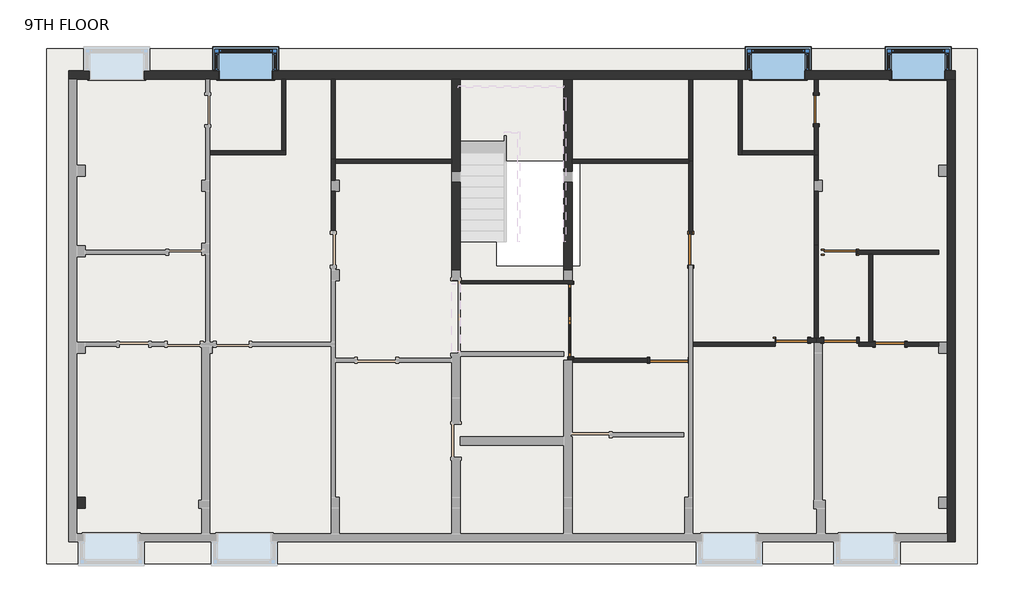
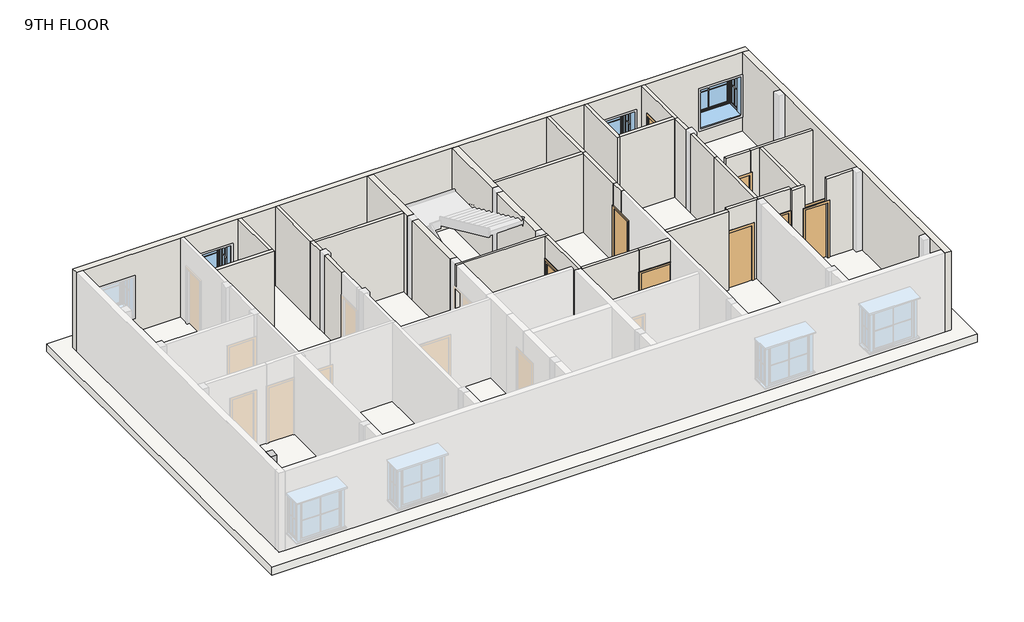
# One storey, part 2 of 3: 34 walls, 8 doors, 3 windows, 1 column, 1 slab.
"""IFC4 building model written with IfcOpenShell, lengths in millimetres."""

from ifc_helpers import new_model, si_unit, frame, origin, place, context, project, spatial, polyline, outline, extrude, faceted_brep, transform, mapped, element, save
from components import door_04ab2522, m_door_single_panel_05506f71, door_85b31ab1, door_1991e9a2, door_a431d384, door_82def9da, m_door_single_panel_3_x7_f8176753, window_19bbd869

model = new_model("IFC4")

# Units and contexts
model_context = context("Model", 3, world=origin())
ifc_project = project(units=[si_unit("LENGTHUNIT", "METRE", prefix="MILLI")], contexts=[model_context])

# Site, building, storey
site = spatial("IfcSite", under=ifc_project)
building = spatial("IfcBuilding", under=site)
storey = spatial("IfcBuildingStorey", under=building, Name="9TH FLOOR", Elevation=32004.0)

# Column
placement = place(None, origin())
element("IfcColumn", 1, ObjectType="Rectangular Column : 1'X 9\"", at=placement, inside=storey, context=model_context, shape_type="SweptSolid", body=[
    extrude(outline(polyline([(-12224.6987957, -3709.2932671), (-12224.6987957, -4014.0932671), (-12453.2987957, -4014.0932671), (-12453.2987957, -3709.2932671), (-12224.6987957, -3709.2932671)])), frame((0.0, 0.0, 32004.0), z_axis=(0.0, 0.0, 1.0), x_axis=(1.0, 0.0, 0.0)), (0.0, 0.0, 1.0), 3048.0),
])

# Doors
door_shape = door_04ab2522(model_context)
element("IfcDoor", 2, ObjectType="M_Door-Double-Glass : 6'7\"X7'", at=placement, inside=storey, context=model_context, shape_type="MappedRepresentation", body=[
    mapped(door_shape, transform((1217.5394962, 1183.3817656, 32004.0), x_axis=(0.0, 1.0, 0.0), y_axis=(-1.0, 0.0, 0.0), z_axis=(0.0, 0.0, 1.0))),
])
m_door_single_panel_shape = m_door_single_panel_05506f71(model_context)
element("IfcDoor", 3, ObjectType="M_Door-Single-Panel", at=placement, inside=storey, context=model_context, shape_type="MappedRepresentation", body=[
    mapped(m_door_single_panel_shape, transform((3933.4813133, 90.9578621, 32004.0), x_axis=(1.0, 0.0, 0.0), y_axis=(0.0, 1.0, 0.0), z_axis=(0.0, 0.0, 1.0))),
])
door_2_shape = door_85b31ab1(model_context)
element("IfcDoor", 4, ObjectType="M_Door-Single-Panel : 2'10\"X7' 2", at=placement, inside=storey, context=model_context, shape_type="MappedRepresentation", body=[
    mapped(door_2_shape, transform((4532.9512082, 3142.9626891, 32004.0), x_axis=(0.0, -1.0, 0.0), y_axis=(1.0, 0.0, 0.0), z_axis=(0.0, 0.0, 1.0))),
])
door_3_shape = door_1991e9a2(model_context)
element("IfcDoor", 5, ObjectType="M_Door-Single-Panel : 2'11\"X7' 3", at=placement, inside=storey, context=model_context, shape_type="MappedRepresentation", body=[
    mapped(door_3_shape, transform((7330.1405552, 640.4567334, 32004.0), x_axis=(1.0, 0.0, 0.0), y_axis=(0.0, 1.0, 0.0), z_axis=(0.0, 0.0, 1.0))),
])
element("IfcDoor", 6, ObjectType="M_Door-Single-Panel : 2'11\"X7' 3", at=placement, inside=storey, context=model_context, shape_type="MappedRepresentation", body=[
    mapped(door_3_shape, transform((8664.274939, 3078.8567332, 32004.0), x_axis=(-1.0, 0.0, 0.0), y_axis=(0.0, -1.0, 0.0), z_axis=(0.0, 0.0, 1.0))),
])
door_4_shape = door_a431d384(model_context)
element("IfcDoor", 7, ObjectType="M_Door-Single-Panel : 2'7\"X7' 2", at=placement, inside=storey, context=model_context, shape_type="MappedRepresentation", body=[
    mapped(door_4_shape, transform((8000.0512079, 7021.3751452, 32004.0), x_axis=(0.0, 1.0, 0.0), y_axis=(-1.0, 0.0, 0.0), z_axis=(0.0, 0.0, 1.0))),
])
door_5_shape = door_82def9da(model_context)
element("IfcDoor", 8, ObjectType="M_Door-Single-Panel : 2'8\"X7'", at=placement, inside=storey, context=model_context, shape_type="MappedRepresentation", body=[
    mapped(door_5_shape, transform((10046.0486694, 526.1567295, 32004.0), x_axis=(-1.0, 0.0, 0.0), y_axis=(0.0, -1.0, 0.0), z_axis=(0.0, 0.0, 1.0))),
])
m_door_single_panel_3_x7_shape = m_door_single_panel_3_x7_f8176753(model_context)
element("IfcDoor", 9, ObjectType="M_Door-Single-Panel : 3'X7'", at=placement, inside=storey, context=model_context, shape_type="MappedRepresentation", body=[
    mapped(m_door_single_panel_3_x7_shape, transform((8666.8012079, 640.4567334, 32004.0), x_axis=(-1.0, 0.0, 0.0), y_axis=(0.0, -1.0, 0.0), z_axis=(0.0, 0.0, 1.0))),
])

# Slab
element("IfcSlab", 10, ObjectType="Generic - 12\"", at=placement, inside=storey, context=model_context, shape_type="SweptSolid", body=[
    extrude(outline(polyline([(12464.1012075, 8698.6067329), (12464.1012075, -5550.7932662), (-13291.4987957, -5550.7932662), (-13291.4987957, 8698.6067329), (12464.1012075, 8698.6067329)]), holes=[polyline([(1456.6270108, 2700.0220048), (1456.6270108, 5595.6220048), (-829.3729892, 5595.6220048), (-829.3729892, 2700.0220048), (1456.6270108, 2700.0220048)])]), frame((0.0, 0.0, 31699.2), z_axis=(0.0, 0.0, 1.0), x_axis=(1.0, 0.0, 0.0)), (0.0, 0.0, 1.0), 304.8),
])

# Walls
element("IfcWall", 11, ObjectType="3.5\"", at=placement, inside=storey, context=model_context, shape_type="Brep", body=[
    faceted_brep([(1272.3082462, 2196.2067742, 35052.0), (1158.0082462, 2196.2067742, 35052.0), (-1848.7987998, 2196.2067742, 35052.0), (-2077.3987998, 2196.2067742, 35052.0), (-2077.3987998, 2196.2067742, 34137.6), (-1848.7987998, 2196.2067742, 34137.6), (-1848.7987998, 2196.2067742, 32004.0), (1158.0082462, 2196.2067742, 32004.0), (1272.3082462, 2196.2067742, 32004.0), (1272.3082462, 2285.1067742, 32004.0), (1253.2582462, 2285.1067742, 32004.0), (1024.6582462, 2285.1067742, 32004.0), (-1845.5417538, 2285.1067742, 32004.0), (-2074.1417538, 2285.1067742, 32004.0), (-2077.3987998, 2285.1067742, 32004.0), (-2077.3987998, 2285.1067742, 35052.0), (-2074.1417538, 2285.1067742, 35052.0), (-1845.5417538, 2285.1067742, 35052.0), (1024.6582462, 2285.1067742, 35052.0), (1253.2582462, 2285.1067742, 35052.0), (1272.3082462, 2285.1067742, 35052.0), (-1848.7987998, 2281.9317742, 32004.0), (-2077.3987998, 2281.9317742, 32004.0), (-2077.3987998, 2281.9317742, 34137.6), (-1848.7987998, 2281.9317742, 34137.6)], [[[0, 1, 2, 3, 4, 5, 6, 7, 8]], [[9, 10, 11, 12, 13, 14, 15, 16, 17, 18, 19, 20]], [[14, 13, 12, 11, 10, 9, 8, 7, 6, 21, 22]], [[3, 2, 1, 0, 20, 19, 18, 17, 16, 15]], [[0, 8, 9, 20]], [[3, 15, 14, 22, 23, 4]], [[24, 21, 6, 5]], [[23, 24, 5, 4]], [[21, 24, 23, 22]]]),
])
element("IfcWall", 12, ObjectType="4.5\"", at=placement, inside=storey, context=model_context, shape_type="SweptSolid", body=[
    extrude(outline(polyline([(3132.0737955, 35052.0), (3628.3344162, 35052.0), (3628.3344162, 32004.0), (3574.7626891, 32004.0), (3574.7626891, 34137.6), (3132.0737955, 34137.6), (3132.0737955, 35052.0)])), frame((4475.8012082, 0.0, 0.0), z_axis=(1.0, 0.0, 0.0), x_axis=(0.0, 1.0, 0.0)), (0.0, 0.0, 1.0), 114.3),
])
element("IfcWall", 13, ObjectType="4.5\"", at=placement, inside=storey, context=model_context, shape_type="Brep", body=[
    faceted_brep([(8000.0512079, 583.3067334, 32004.0), (8000.0512079, 583.3067334, 35052.0), (7942.9012047, 583.3067334, 35052.0), (6862.7668241, 583.3067334, 35052.0), (6862.7668241, 583.3067334, 32004.0), (6885.6405552, 583.3067334, 32004.0), (6885.6405552, 583.3067334, 34137.6), (7774.6405552, 583.3067334, 34137.6), (7774.6405552, 583.3067334, 32004.0), (7942.9012047, 583.3067334, 32004.0), (8000.0512079, 697.6067334, 35052.0), (8000.0512079, 697.6067334, 32004.0), (7942.9012079, 697.6067334, 32004.0), (7774.6405552, 697.6067334, 32004.0), (7774.6405552, 697.6067334, 34137.6), (6885.6405552, 697.6067334, 34137.6), (6885.6405552, 697.6067334, 32004.0), (6862.7668241, 697.6067334, 32004.0), (6862.7668241, 697.6067334, 35052.0), (7942.9012079, 697.6067334, 35052.0)], [[[0, 1, 2, 3, 4, 5, 6, 7, 8, 9]], [[10, 11, 12, 13, 14, 15, 16, 17, 18, 19]], [[4, 17, 16, 5]], [[11, 0, 9, 8, 13, 12]], [[1, 0, 11, 10]], [[3, 2, 1, 10, 19, 18]], [[4, 3, 18, 17]], [[7, 14, 13, 8]], [[14, 7, 6, 15]], [[15, 6, 5, 16]]]),
])
element("IfcWall", 14, ObjectType="4.5\"", at=placement, inside=storey, context=model_context, shape_type="Brep", body=[
    faceted_brep([(9187.5012047, 583.3067334, 32004.0), (9187.5012047, 583.3067334, 35052.0), (8171.5012047, 583.3067334, 35052.0), (8000.0512079, 583.3067334, 35052.0), (8000.0512079, 583.3067334, 32004.0), (8171.5012047, 583.3067334, 32004.0), (8209.6012079, 583.3067334, 32004.0), (8209.6012079, 583.3067334, 34137.6), (9124.0012079, 583.3067334, 34137.6), (9124.0012079, 583.3067334, 32004.0), (9187.5012047, 697.6067334, 35052.0), (9187.5012047, 697.6067334, 32004.0), (9124.0012079, 697.6067334, 32004.0), (9124.0012079, 697.6067334, 34137.6), (8209.6012079, 697.6067334, 34137.6), (8209.6012079, 697.6067334, 32004.0), (8057.2012079, 697.6067334, 32004.0), (8000.0512079, 697.6067334, 32004.0), (8000.0512079, 697.6067334, 35052.0), (8057.2012079, 697.6067334, 35052.0)], [[[0, 1, 2, 3, 4, 5, 6, 7, 8, 9]], [[10, 11, 12, 13, 14, 15, 16, 17, 18, 19]], [[11, 0, 9, 12]], [[4, 17, 16, 15, 6, 5]], [[1, 0, 11, 10]], [[3, 2, 1, 10, 19, 18]], [[4, 3, 18, 17]], [[7, 14, 13, 8]], [[8, 13, 12, 9]], [[14, 7, 6, 15]]]),
])
element("IfcWall", 15, ObjectType="4.5\"", at=placement, inside=storey, context=model_context, shape_type="SweptSolid", body=[
    extrude(outline(polyline([(32004.0, 9131.6486701), (35052.0, 9131.6486701), (35052.0, 8245.174939), (34137.6, 8245.174939), (34137.6, 9108.774939), (32004.0, 9108.774939), (32004.0, 9131.6486701)])), frame((0.0, 3021.7067332, 0.0), z_axis=(0.0, 1.0, 0.0), x_axis=(0.0, 0.0, 1.0)), (0.0, 0.0, 1.0), 114.3),
])
element("IfcWall", 16, ObjectType="4.5\"", at=placement, inside=storey, context=model_context, shape_type="Brep", body=[
    faceted_brep([(7942.9012079, 5764.9067329, 35052.0), (7942.9012079, 5879.2067329, 35052.0), (7942.9012079, 7860.4067329, 35052.0), (7942.9012079, 7860.4067329, 32004.0), (7942.9012079, 7415.0751452, 32004.0), (7942.9012079, 7415.0751452, 34137.6), (7942.9012079, 6627.6751452, 34137.6), (7942.9012079, 6627.6751452, 32004.0), (7942.9012079, 5879.2067329, 32004.0), (7942.9012079, 5764.9067329, 32004.0), (8057.2012079, 7860.4067329, 35052.0), (8057.2012079, 5764.9067329, 35052.0), (8057.2012079, 5764.9067329, 32004.0), (8057.2012079, 6627.6751452, 32004.0), (8057.2012079, 6627.6751452, 34137.6), (8057.2012079, 7415.0751452, 34137.6), (8057.2012079, 7415.0751452, 32004.0), (8057.2012079, 7860.4067329, 32004.0)], [[[0, 1, 2, 3, 4, 5, 6, 7, 8, 9]], [[10, 11, 12, 13, 14, 15, 16, 17]], [[12, 9, 8, 7, 13]], [[3, 17, 16, 4]], [[2, 1, 0, 11, 10]], [[15, 5, 4, 16]], [[5, 15, 14, 6]], [[6, 14, 13, 7]], [[0, 9, 12, 11]], [[3, 2, 10, 17]]]),
])
element("IfcWall", 17, ObjectType="4.5\"", at=placement, inside=storey, context=model_context, shape_type="SweptSolid", body=[
    extrude(outline(polyline([(34137.6, 4466.8813133), (32004.0, 4466.8813133), (32004.0, 4475.8012082), (35052.0, 4475.8012082), (35052.0, 3334.0114184), (32004.0, 3334.0114184), (32004.0, 3400.0813133), (34137.6, 3400.0813133), (34137.6, 4466.8813133)])), frame((0.0, 33.8078621, 0.0), z_axis=(0.0, 1.0, 0.0), x_axis=(0.0, 0.0, 1.0)), (0.0, 0.0, 1.0), 114.3),
])
element("IfcWall", 18, ObjectType="4.5\"", at=placement, inside=storey, context=model_context, shape_type="Brep", body=[
    faceted_brep([(1158.0082462, 2196.2067742, 32004.0), (1158.0082462, 2186.6817656, 32004.0), (1158.0082462, 2186.6817656, 34137.6), (1158.0082462, 180.0817656, 34137.6), (1158.0082462, 180.0817656, 32004.0), (1158.0082462, 90.9578621, 32004.0), (1158.0082462, 90.9578621, 35052.0), (1158.0082462, 2196.2067742, 35052.0), (1272.3082462, 2186.6817656, 34137.6), (1272.3082462, 2186.6817656, 32004.0), (1272.3082462, 2196.2067742, 32004.0), (1272.3082462, 2196.2067742, 35052.0), (1272.3082462, 148.1078621, 35052.0), (1272.3082462, 90.9578621, 35052.0), (1272.3082462, 90.9578621, 32004.0), (1272.3082462, 148.1078621, 32004.0), (1272.3082462, 180.0817656, 32004.0), (1272.3082462, 180.0817656, 34137.6), (1250.0012085, 90.9578621, 32004.0), (1250.0012085, 90.9578621, 35052.0)], [[[0, 1, 2, 3, 4, 5, 6, 7]], [[8, 9, 10, 11, 12, 13, 14, 15, 16, 17]], [[10, 9, 1, 0]], [[16, 15, 14, 18, 5, 4]], [[6, 5, 18, 14, 13, 19]], [[7, 6, 19, 13, 12, 11]], [[0, 7, 11, 10]], [[2, 1, 9, 8]], [[3, 2, 8, 17]], [[4, 3, 17, 16]]]),
])
element("IfcWall", 19, ObjectType="4.5\"", at=placement, inside=storey, context=model_context, shape_type="Brep", body=[
    faceted_brep([(1250.0012085, 5536.3067329, 32004.0), (4475.8012082, 5536.3067329, 32004.0), (4475.8012082, 5536.3067329, 35052.0), (1250.0012085, 5536.3067329, 35052.0), (1250.0012085, 5650.6067329, 32004.0), (1250.0012085, 5650.6067329, 35052.0), (4475.8012082, 5650.6067329, 35052.0), (4475.8012082, 5650.6067329, 32004.0), (4475.8012082, 5593.4567329, 32004.0), (4475.8012082, 5593.4567329, 35052.0)], [[[0, 1, 2, 3]], [[4, 5, 6, 7]], [[1, 0, 4, 7, 8]], [[3, 2, 9, 6, 5]], [[2, 1, 8, 7, 6, 9]], [[0, 3, 5, 4]]]),
])
element("IfcWall", 20, ObjectType="4.5\"", at=placement, inside=storey, context=model_context, shape_type="Brep", body=[
    faceted_brep([(8057.2012047, 3270.1432417, 32004.0), (8057.2012047, 4760.6824989, 32004.0), (8057.2012047, 4760.6824989, 35052.0), (8057.2012047, 3270.1432417, 35052.0), (7942.9012047, 3270.1432417, 32004.0), (7942.9012047, 3270.1432417, 35052.0), (7942.9012047, 4760.6824989, 35052.0), (7942.9012047, 4760.6824989, 32004.0), (7943.9040565, 4760.6824989, 32004.0), (7943.9040565, 4760.6824989, 35052.0)], [[[0, 1, 2, 3]], [[4, 5, 6, 7]], [[1, 0, 4, 7, 8]], [[2, 1, 8, 7, 6, 9]], [[3, 2, 9, 6, 5]], [[0, 3, 5, 4]]]),
])
element("IfcWall", 21, ObjectType="4.5\"", at=placement, inside=storey, context=model_context, shape_type="Brep", body=[
    faceted_brep([(7942.9012079, 3270.1432417, 32004.0), (7942.9012079, 697.6067334, 32004.0), (7942.9012079, 697.6067334, 35052.0), (7942.9012079, 3270.1432417, 35052.0), (8057.2012079, 3270.1432417, 32004.0), (8057.2012079, 3270.1432417, 35052.0), (8057.2012079, 697.6067334, 35052.0), (8057.2012079, 697.6067334, 32004.0), (8000.0512079, 697.6067334, 32004.0), (8000.0512079, 697.6067334, 35052.0)], [[[0, 1, 2, 3]], [[4, 5, 6, 7]], [[1, 0, 4, 7, 8]], [[3, 2, 9, 6, 5]], [[0, 3, 5, 4]], [[2, 1, 8, 7, 6, 9]]]),
])
element("IfcWall", 22, ObjectType="4.5\"", at=placement, inside=storey, context=model_context, shape_type="SweptSolid", body=[
    extrude(outline(polyline([(8058.2040565, 5763.9824989), (8058.2040565, 5065.4824989), (7943.9040565, 5065.4824989), (7943.9040565, 5763.9824989), (8058.2040565, 5763.9824989)])), frame((0.0, 0.0, 32004.0), z_axis=(0.0, 0.0, 1.0), x_axis=(1.0, 0.0, 0.0)), (0.0, 0.0, 1.0), 3048.0),
])
element("IfcWall", 23, ObjectType="4.5\"", at=placement, inside=storey, context=model_context, shape_type="SweptSolid", body=[
    extrude(outline(polyline([(1272.3082462, 148.1078621), (3334.0114184, 148.1078621), (3334.0114184, 33.8078621), (1250.0012085, 33.8078621), (1250.0012085, 90.9578621), (1272.3082462, 90.9578621), (1272.3082462, 148.1078621)])), frame((0.0, 0.0, 32004.0), z_axis=(0.0, 0.0, 1.0), x_axis=(1.0, 0.0, 0.0)), (0.0, 0.0, 1.0), 3048.0),
])
element("IfcWall", 24, ObjectType="4.5\" 2", at=placement, inside=storey, context=model_context, shape_type="Brep", body=[
    faceted_brep([(-8770.2987992, 5764.9067329, 32004.0), (-6674.7987994, 5764.9067329, 32004.0), (-6674.7987994, 5764.9067329, 35052.0), (-8770.2987992, 5764.9067329, 35052.0), (-8770.2987992, 5879.2067329, 32004.0), (-8770.2987992, 5879.2067329, 35052.0), (-6789.0987994, 5879.2067329, 35052.0), (-6674.7987994, 5879.2067329, 35052.0), (-6674.7987994, 5879.2067329, 32004.0), (-6789.0987994, 5879.2067329, 32004.0)], [[[0, 1, 2, 3]], [[4, 5, 6, 7, 8, 9]], [[1, 0, 4, 9, 8]], [[3, 2, 7, 6, 5]], [[0, 3, 5, 4]], [[2, 1, 8, 7]]]),
])
element("IfcWall", 25, ObjectType="4.5\" 2", at=placement, inside=storey, context=model_context, shape_type="SweptSolid", body=[
    extrude(outline(polyline([(-6674.7987994, 7860.4067329), (-6674.7987994, 5879.2067329), (-6789.0987994, 5879.2067329), (-6789.0987994, 7860.4067329), (-6674.7987994, 7860.4067329)])), frame((0.0, 0.0, 32004.0), z_axis=(0.0, 0.0, 1.0), x_axis=(1.0, 0.0, 0.0)), (0.0, 0.0, 1.0), 3048.0),
])
element("IfcWall", 26, ObjectType="4.5\" 2", at=placement, inside=storey, context=model_context, shape_type="SweptSolid", body=[
    extrude(outline(polyline([(-5303.1987995, 4761.606733), (-5303.1987995, 3671.8272228), (-5417.4987995, 3671.8272228), (-5417.4987995, 4761.606733), (-5303.1987995, 4761.606733)])), frame((0.0, 0.0, 32004.0), z_axis=(0.0, 0.0, 1.0), x_axis=(1.0, 0.0, 0.0)), (0.0, 0.0, 1.0), 3048.0),
])
element("IfcWall", 27, ObjectType="4.5\" 2", at=placement, inside=storey, context=model_context, shape_type="Brep", body=[
    faceted_brep([(-5303.1987995, 5066.406733, 32004.0), (-5303.1987995, 5536.3067329, 32004.0), (-5303.1987995, 5650.6067329, 32004.0), (-5303.1987995, 5650.6067329, 35052.0), (-5303.1987995, 5536.3067329, 35052.0), (-5303.1987995, 5066.406733, 35052.0), (-5417.4987995, 5066.406733, 32004.0), (-5417.4987995, 5066.406733, 35052.0), (-5417.4987995, 5650.6067329, 35052.0), (-5417.4987995, 5650.6067329, 32004.0)], [[[0, 1, 2, 3, 4, 5]], [[6, 7, 8, 9]], [[2, 1, 0, 6, 9]], [[5, 4, 3, 8, 7]], [[0, 5, 7, 6]], [[3, 2, 9, 8]]]),
])
element("IfcWall", 28, ObjectType="4.5\" 2", at=placement, inside=storey, context=model_context, shape_type="SweptSolid", body=[
    extrude(outline(polyline([(-2077.3987998, 5536.3067329), (-5303.1987995, 5536.3067329), (-5303.1987995, 5650.6067329), (-2077.3987998, 5650.6067329), (-2077.3987998, 5536.3067329)])), frame((0.0, 0.0, 32004.0), z_axis=(0.0, 0.0, 1.0), x_axis=(1.0, 0.0, 0.0)), (0.0, 0.0, 1.0), 3048.0),
])
element("IfcWall", 29, ObjectType="4.5\" 2", at=placement, inside=storey, context=model_context, shape_type="SweptSolid", body=[
    extrude(outline(polyline([(-5417.4987995, 5650.6067329), (-5417.4987995, 7860.4067329), (-5303.1987995, 7860.4067329), (-5303.1987995, 5650.6067329), (-5417.4987995, 5650.6067329)])), frame((0.0, 0.0, 32004.0), z_axis=(0.0, 0.0, 1.0), x_axis=(1.0, 0.0, 0.0)), (0.0, 0.0, 1.0), 3048.0),
])
element("IfcWall", 30, ObjectType="4.5\" 2", at=placement, inside=storey, context=model_context, shape_type="Brep", body=[
    faceted_brep([(4475.8012082, 5593.4567329, 32004.0), (4475.8012082, 5536.3067329, 32004.0), (4475.8012082, 3628.3344162, 32004.0), (4475.8012082, 3628.3344162, 35052.0), (4475.8012082, 5536.3067329, 35052.0), (4475.8012082, 5593.4567329, 35052.0), (4590.1012082, 5593.4567329, 32004.0), (4590.1012082, 5593.4567329, 35052.0), (4590.1012082, 3628.3344162, 35052.0), (4590.1012082, 3628.3344162, 32004.0)], [[[0, 1, 2, 3, 4, 5]], [[6, 7, 8, 9]], [[2, 1, 0, 6, 9]], [[3, 2, 9, 8]], [[5, 4, 3, 8, 7]], [[0, 5, 7, 6]]]),
])
element("IfcWall", 31, ObjectType="4.5\" 2", at=placement, inside=storey, context=model_context, shape_type="SweptSolid", body=[
    extrude(outline(polyline([(6862.7668241, 469.0067334), (4590.1012082, 469.0067334), (4590.1012082, 583.3067334), (6862.7668241, 583.3067334), (6862.7668241, 469.0067334)])), frame((0.0, 0.0, 32004.0), z_axis=(0.0, 0.0, 1.0), x_axis=(1.0, 0.0, 0.0)), (0.0, 0.0, 1.0), 3048.0),
])
element("IfcWall", 32, ObjectType="4.5\" 2", at=placement, inside=storey, context=model_context, shape_type="Brep", body=[
    faceted_brep([(9182.4486694, 469.0067295, 32004.0), (9639.6486694, 469.0067295, 32004.0), (9639.6486694, 469.0067295, 35052.0), (9182.4486694, 469.0067295, 35052.0), (9182.4486694, 583.3067295, 32004.0), (9182.4486694, 583.3067295, 35052.0), (9451.1098918, 583.3067295, 35052.0), (9565.4098918, 583.3067295, 35052.0), (9639.6486694, 583.3067295, 35052.0), (9639.6486694, 583.3067295, 32004.0), (9565.4098918, 583.3067295, 32004.0), (9451.1098918, 583.3067295, 32004.0)], [[[0, 1, 2, 3]], [[4, 5, 6, 7, 8, 9, 10, 11]], [[1, 0, 4, 11, 10, 9]], [[2, 1, 9, 8]], [[3, 2, 8, 7, 6, 5]], [[0, 3, 5, 4]]]),
])
element("IfcWall", 33, ObjectType="4.5\" 2", at=placement, inside=storey, context=model_context, shape_type="SweptSolid", body=[
    extrude(outline(polyline([(32004.0, 11397.3012075), (35052.0, 11397.3012075), (35052.0, 10443.8236977), (34137.6, 10443.8236977), (34137.6, 10452.4486694), (32004.0, 10452.4486694), (32004.0, 11397.3012075)])), frame((0.0, 469.0067295, 0.0), z_axis=(0.0, 1.0, 0.0), x_axis=(0.0, 0.0, 1.0)), (0.0, 0.0, 1.0), 114.3),
])
element("IfcWall", 34, ObjectType="4.5\" 2", at=placement, inside=storey, context=model_context, shape_type="SweptSolid", body=[
    extrude(outline(polyline([(9565.4098918, 3021.7067332), (9565.4098918, 583.3067295), (9451.1098918, 583.3067295), (9451.1098918, 3021.7067332), (9565.4098918, 3021.7067332)])), frame((0.0, 0.0, 32004.0), z_axis=(0.0, 0.0, 1.0), x_axis=(1.0, 0.0, 0.0)), (0.0, 0.0, 1.0), 3048.0),
])
element("IfcWall", 35, ObjectType="4.5\" 2", at=placement, inside=storey, context=model_context, shape_type="Brep", body=[
    faceted_brep([(9131.6486701, 3021.7067332, 32004.0), (9451.1098918, 3021.7067332, 32004.0), (9565.4098918, 3021.7067332, 32004.0), (11397.3012075, 3021.7067332, 32004.0), (11397.3012075, 3021.7067332, 35052.0), (9565.4098918, 3021.7067332, 35052.0), (9451.1098918, 3021.7067332, 35052.0), (9131.6486701, 3021.7067332, 35052.0), (9131.6486701, 3136.0067332, 32004.0), (9131.6486701, 3136.0067332, 35052.0), (11397.3012075, 3136.0067332, 35052.0), (11397.3012075, 3136.0067332, 32004.0)], [[[0, 1, 2, 3, 4, 5, 6, 7]], [[8, 9, 10, 11]], [[3, 2, 1, 0, 8, 11]], [[4, 3, 11, 10]], [[7, 6, 5, 4, 10, 9]], [[0, 7, 9, 8]]]),
])
element("IfcWall", 36, ObjectType="4.5\" 2", at=placement, inside=storey, context=model_context, shape_type="Brep", body=[
    faceted_brep([(4590.1012082, 5593.4567329, 32004.0), (4590.1012082, 7860.4067329, 32004.0), (4590.1012082, 7860.4067329, 35052.0), (4590.1012082, 5593.4567329, 35052.0), (4475.8012082, 5593.4567329, 32004.0), (4475.8012082, 5593.4567329, 35052.0), (4475.8012082, 5650.6067329, 35052.0), (4475.8012082, 7860.4067329, 35052.0), (4475.8012082, 7860.4067329, 32004.0), (4475.8012082, 5650.6067329, 32004.0)], [[[0, 1, 2, 3]], [[4, 5, 6, 7, 8, 9]], [[1, 0, 4, 9, 8]], [[3, 2, 7, 6, 5]], [[0, 3, 5, 4]], [[2, 1, 8, 7]]]),
])
element("IfcWall", 37, ObjectType="4.5\" 2", at=placement, inside=storey, context=model_context, shape_type="Brep", body=[
    faceted_brep([(5847.401208, 7860.4067329, 32004.0), (5847.401208, 5764.9067329, 32004.0), (5847.401208, 5764.9067329, 35052.0), (5847.401208, 7860.4067329, 35052.0), (5961.701208, 7860.4067329, 32004.0), (5961.701208, 7860.4067329, 35052.0), (5961.701208, 5879.2067329, 35052.0), (5961.701208, 5764.9067329, 35052.0), (5961.701208, 5764.9067329, 32004.0), (5961.701208, 5879.2067329, 32004.0)], [[[0, 1, 2, 3]], [[4, 5, 6, 7, 8, 9]], [[1, 0, 4, 9, 8]], [[3, 2, 7, 6, 5]], [[2, 1, 8, 7]], [[0, 3, 5, 4]]]),
])
element("IfcWall", 38, ObjectType="4.5\" 2", at=placement, inside=storey, context=model_context, shape_type="SweptSolid", body=[
    extrude(outline(polyline([(7942.9012079, 5764.9067329), (5961.701208, 5764.9067329), (5961.701208, 5879.2067329), (7942.9012079, 5879.2067329), (7942.9012079, 5764.9067329)])), frame((0.0, 0.0, 32004.0), z_axis=(0.0, 0.0, 1.0), x_axis=(1.0, 0.0, 0.0)), (0.0, 0.0, 1.0), 3048.0),
])
element("IfcWall", 39, ObjectType="9\"", at=placement, inside=storey, context=model_context, shape_type="Brep", body=[
    faceted_brep([(-12681.8987957, 7860.4067329, 32004.0), (-12453.2987957, 7860.4067329, 32004.0), (-8884.5987992, 7860.4067329, 32004.0), (-8770.2987992, 7860.4067329, 32004.0), (-6789.0987994, 7860.4067329, 32004.0), (-6674.7987994, 7860.4067329, 32004.0), (-5417.4987995, 7860.4067329, 32004.0), (-5303.1987995, 7860.4067329, 32004.0), (-2074.1417538, 7860.4067329, 32004.0), (-1845.5417538, 7860.4067329, 32004.0), (1021.4012085, 7860.4067329, 32004.0), (1250.0012085, 7860.4067329, 32004.0), (4475.8012082, 7860.4067329, 32004.0), (4590.1012082, 7860.4067329, 32004.0), (5847.401208, 7860.4067329, 32004.0), (5961.701208, 7860.4067329, 32004.0), (7942.9012079, 7860.4067329, 32004.0), (8057.2012079, 7860.4067329, 32004.0), (11625.9012075, 7860.4067329, 32004.0), (11854.5012075, 7860.4067329, 32004.0), (11854.5012075, 7860.4067329, 35052.0), (11625.9012075, 7860.4067329, 35052.0), (8057.2012079, 7860.4067329, 35052.0), (7942.9012079, 7860.4067329, 35052.0), (5961.701208, 7860.4067329, 35052.0), (5847.401208, 7860.4067329, 35052.0), (4590.1012082, 7860.4067329, 35052.0), (4475.8012082, 7860.4067329, 35052.0), (1250.0012085, 7860.4067329, 35052.0), (1021.4012085, 7860.4067329, 35052.0), (-1845.5417538, 7860.4067329, 35052.0), (-2074.1417538, 7860.4067329, 35052.0), (-5303.1987995, 7860.4067329, 35052.0), (-5417.4987995, 7860.4067329, 35052.0), (-6674.7987994, 7860.4067329, 35052.0), (-6789.0987994, 7860.4067329, 35052.0), (-8770.2987992, 7860.4067329, 35052.0), (-8884.5987992, 7860.4067329, 35052.0), (-12453.2987957, 7860.4067329, 35052.0), (-12681.8987957, 7860.4067329, 35052.0), (11575.8012075, 7860.4067329, 34154.8), (11575.8012075, 7860.4067329, 32604.0), (10075.8012075, 7860.4067329, 32604.0), (10075.8012075, 7860.4067329, 34154.8), (7702.301208, 7860.4067329, 34154.8), (7702.301208, 7860.4067329, 32604.0), (6202.301208, 7860.4067329, 32604.0), (6202.301208, 7860.4067329, 34154.8), (-7029.6987993, 7860.4067329, 34154.8), (-7029.6987993, 7860.4067329, 32604.0), (-8529.6987993, 7860.4067329, 32604.0), (-8529.6987993, 7860.4067329, 34154.8), (-10598.3987957, 7860.4067329, 34154.8), (-10598.3987957, 7860.4067329, 32604.0), (-12098.3987957, 7860.4067329, 32604.0), (-12098.3987957, 7860.4067329, 34154.8), (-12681.8987957, 8089.0067329, 32004.0), (-12681.8987957, 8089.0067329, 35052.0), (11854.5012075, 8089.0067329, 35052.0), (11854.5012075, 8089.0067329, 32004.0), (11575.8012075, 8089.0067329, 34154.8), (10075.8012075, 8089.0067329, 34154.8), (10075.8012075, 8089.0067329, 32604.0), (11575.8012075, 8089.0067329, 32604.0), (7702.301208, 8089.0067329, 34154.8), (6202.301208, 8089.0067329, 34154.8), (6202.301208, 8089.0067329, 32604.0), (7702.301208, 8089.0067329, 32604.0), (-7029.6987993, 8089.0067329, 34154.8), (-8529.6987993, 8089.0067329, 34154.8), (-8529.6987993, 8089.0067329, 32604.0), (-7029.6987993, 8089.0067329, 32604.0), (-10598.3987957, 8089.0067329, 34154.8), (-12098.3987957, 8089.0067329, 34154.8), (-12098.3987957, 8089.0067329, 32604.0), (-10598.3987957, 8089.0067329, 32604.0)], [[[0, 1, 2, 3, 4, 5, 6, 7, 8, 9, 10, 11, 12, 13, 14, 15, 16, 17, 18, 19, 20, 21, 22, 23, 24, 25, 26, 27, 28, 29, 30, 31, 32, 33, 34, 35, 36, 37, 38, 39], [40, 41, 42, 43], [44, 45, 46, 47], [48, 49, 50, 51], [52, 53, 54, 55]], [[56, 57, 58, 59], [60, 61, 62, 63], [64, 65, 66, 67], [68, 69, 70, 71], [72, 73, 74, 75]], [[19, 18, 17, 16, 15, 14, 13, 12, 11, 10, 9, 8, 7, 6, 5, 4, 3, 2, 1, 0, 56, 59]], [[39, 38, 37, 36, 35, 34, 33, 32, 31, 30, 29, 28, 27, 26, 25, 24, 23, 22, 21, 20, 58, 57]], [[20, 19, 59, 58]], [[0, 39, 57, 56]], [[41, 40, 60, 63]], [[42, 41, 63, 62]], [[43, 42, 62, 61]], [[40, 43, 61, 60]], [[45, 44, 64, 67]], [[46, 45, 67, 66]], [[47, 46, 66, 65]], [[44, 47, 65, 64]], [[49, 48, 68, 71]], [[50, 49, 71, 70]], [[51, 50, 70, 69]], [[48, 51, 69, 68]], [[53, 52, 72, 75]], [[54, 53, 75, 74]], [[55, 54, 74, 73]], [[52, 55, 73, 72]]]),
])
element("IfcWall", 40, ObjectType="9\"", at=placement, inside=storey, context=model_context, shape_type="Brep", body=[
    faceted_brep([(11625.9012075, 7860.4067329, 32004.0), (11625.9012075, 5479.1567329, 32004.0), (11625.9012075, 5174.3567329, 32004.0), (11625.9012075, 583.3067295, 32004.0), (11625.9012075, 278.5067295, 32004.0), (11625.9012075, -3709.2932671, 32004.0), (11625.9012075, -4014.0932671, 32004.0), (11625.9012075, -4712.5932662, 32004.0), (11625.9012075, -4941.1932662, 32004.0), (11625.9012075, -4941.1932662, 35052.0), (11625.9012075, -4712.5932662, 35052.0), (11625.9012075, -4014.0932671, 35052.0), (11625.9012075, -3709.2932671, 35052.0), (11625.9012075, 278.5067295, 35052.0), (11625.9012075, 583.3067295, 35052.0), (11625.9012075, 5174.3567329, 35052.0), (11625.9012075, 5479.1567329, 35052.0), (11625.9012075, 7860.4067329, 35052.0), (11854.5012075, 7860.4067329, 32004.0), (11854.5012075, 7860.4067329, 35052.0), (11854.5012075, -4941.1932662, 35052.0), (11854.5012075, -4941.1932662, 32004.0)], [[[0, 1, 2, 3, 4, 5, 6, 7, 8, 9, 10, 11, 12, 13, 14, 15, 16, 17]], [[18, 19, 20, 21]], [[8, 7, 6, 5, 4, 3, 2, 1, 0, 18, 21]], [[17, 16, 15, 14, 13, 12, 11, 10, 9, 20, 19]], [[0, 17, 19, 18]], [[9, 8, 21, 20]]]),
])
element("IfcWall", 41, ObjectType="9\"", at=placement, inside=storey, context=model_context, shape_type="SweptSolid", body=[
    extrude(outline(polyline([(-2074.1417538, 5320.4067329), (-2074.1417538, 7860.4067329), (-1845.5417538, 7860.4067329), (-1845.5417538, 5320.4067329), (-2074.1417538, 5320.4067329)])), frame((0.0, 0.0, 32004.0), z_axis=(0.0, 0.0, 1.0), x_axis=(1.0, 0.0, 0.0)), (0.0, 0.0, 1.0), 3048.0),
])
element("IfcWall", 42, ObjectType="9\"", at=placement, inside=storey, context=model_context, shape_type="SweptSolid", body=[
    extrude(outline(polyline([(-2074.1417538, 2589.906774), (-2074.1417538, 5015.606774), (-1845.5417538, 5015.606774), (-1845.5417538, 2589.906774), (-2074.1417538, 2589.906774)])), frame((0.0, 0.0, 32004.0), z_axis=(0.0, 0.0, 1.0), x_axis=(1.0, 0.0, 0.0)), (0.0, 0.0, 1.0), 3048.0),
])
element("IfcWall", 43, ObjectType="9\"", at=placement, inside=storey, context=model_context, shape_type="Brep", body=[
    faceted_brep([(1021.4012085, 7860.4067329, 32004.0), (1021.4012085, 5320.4067329, 32004.0), (1021.4012085, 5320.4067329, 35052.0), (1021.4012085, 7860.4067329, 35052.0), (1250.0012085, 7860.4067329, 32004.0), (1250.0012085, 7860.4067329, 35052.0), (1250.0012085, 5650.6067329, 35052.0), (1250.0012085, 5536.3067329, 35052.0), (1250.0012085, 5320.4067329, 35052.0), (1250.0012085, 5320.4067329, 32004.0), (1250.0012085, 5536.3067329, 32004.0), (1250.0012085, 5650.6067329, 32004.0)], [[[0, 1, 2, 3]], [[4, 5, 6, 7, 8, 9, 10, 11]], [[1, 0, 4, 11, 10, 9]], [[2, 1, 9, 8]], [[3, 2, 8, 7, 6, 5]], [[0, 3, 5, 4]]]),
])
element("IfcWall", 44, ObjectType="9\"", at=placement, inside=storey, context=model_context, shape_type="Brep", body=[
    faceted_brep([(1021.4012085, 5015.6067329, 32004.0), (1021.4012085, 2589.9067742, 32004.0), (1021.4012085, 2589.9067742, 35052.0), (1021.4012085, 5015.6067329, 35052.0), (1250.0012085, 5015.6067329, 32004.0), (1250.0012085, 5015.6067329, 35052.0), (1250.0012085, 2589.9067742, 35052.0), (1250.0012085, 2589.9067742, 32004.0), (1024.6582462, 2589.9067742, 32004.0), (1024.6582462, 2589.9067742, 35052.0)], [[[0, 1, 2, 3]], [[4, 5, 6, 7]], [[1, 0, 4, 7, 8]], [[2, 1, 8, 7, 6, 9]], [[3, 2, 9, 6, 5]], [[0, 3, 5, 4]]]),
])

# Windows
window_shape = window_19bbd869(model_context)
element("IfcWindow", 45, ObjectType="4'.8\"x3'.8\"", at=placement, inside=storey, context=model_context, shape_type="MappedRepresentation", body=[
    mapped(window_shape, transform((-7779.6987993, 7974.7067329, 32004.0), x_axis=(1.0, 0.0, 0.0), y_axis=(0.0, 1.0, 0.0), z_axis=(0.0, 0.0, 1.0))),
])
element("IfcWindow", 46, ObjectType="4'.8\"x3'.8\"", at=placement, inside=storey, context=model_context, shape_type="MappedRepresentation", body=[
    mapped(window_shape, transform((6952.301208, 7974.7067329, 32004.0), x_axis=(1.0, 0.0, 0.0), y_axis=(0.0, 1.0, 0.0), z_axis=(0.0, 0.0, 1.0))),
])
element("IfcWindow", 47, ObjectType="4'.8\"x3'.8\"", at=placement, inside=storey, context=model_context, shape_type="MappedRepresentation", body=[
    mapped(window_shape, transform((10825.8012075, 7974.7067329, 32004.0), x_axis=(1.0, 0.0, 0.0), y_axis=(0.0, 1.0, 0.0), z_axis=(0.0, 0.0, 1.0))),
])

save(model, "model.ifc")

# Revit data of these elements
# Type "Rectangular Column : 1'X 9\""
#   Assembly Code = "B1010200"
#   Depth = 1' - 0"
#   Offset Base = 0' - 0"
#   Offset Top = 0' - 0"
#   Width = 0' - 9"
#   Material = none
# Type "M_Door-Double-Glass : 6'7\"X7'"
#   Type Mark = "16"
#   Construction Type Id = "opn-d45"
#   Assembly Code = "C1020"
#   Analytic Construction = "Wood frame, double glass door "
#   W = 3' - 3 1/2"
#   Thickness = 0' - 1.9685"
#   Thermal Resistance (R) = 1.8150 (h·ft²·°F)/BTU
#   Swing Angle [instance default] = 90.00°
#   Heat Transfer Coefficient (U) = 0.5510 BTU/(h·ft²·°F)
#   Height = 7' - 0"
#   Bottom Rail = 0' - 3.93701"
#   Top Rail = 0' - 3.93701"
#   Stiles = 0' - 3.93701"
#   Trim Projection = 0' - 0.98425"
#   Trim Width = 0' - 3.14961"
#   Width = 6' - 7"
#   Define Thermal Properties by = 1
#   Glazing = Glass
#   Panel Material = Wood - Birch - Solid Stained Light Low Gloss
#   Trim Material = Paint - Sienna
#   Visual Light Transmittance = 0
#   Solar Heat Gain Coefficient = 0
#   Function = (empty or 0)
#   Wall Closure = (empty or 0)
# Type "M_Door-Single-Panel"
#   Type Mark = "14"
#   Construction Type Id = "DOOR"
#   Assembly Code = "C1020300"
#   Analytic Construction = "Wooden"
#   Thickness = 0' - 1.9685"
#   Thermal Resistance (R) = 2.5876 (h·ft²·°F)/BTU
#   Swing Angle [instance default] = 90.00°
#   Heat Transfer Coefficient (U) = 0.3865 BTU/(h·ft²·°F)
#   Height = 7' - 0"
#   Trim Projection Ext = 0' - 0.98425"
#   Trim Projection Int = 0' - 0.98425"
#   Trim Width = 0' - 3.14961"
#   Width = 3' - 6"
#   Define Thermal Properties by = 1
#   Panel Material = Wood - Birch - Solid Stained Light Low Gloss
#   Trim Material = Paint - Sienna
#   Visual Light Transmittance = 0
#   Solar Heat Gain Coefficient = 0
#   Function = (empty or 0)
#   Wall Closure = (empty or 0)
# Type "M_Door-Single-Panel : 2'10\"X7' 2"
#   Type Mark = "10"
#   Construction Type Id = "DOOR"
#   Assembly Code = "C1020300"
#   Analytic Construction = "Wooden"
#   Thickness = 0' - 1.9685"
#   Thermal Resistance (R) = 2.5876 (h·ft²·°F)/BTU
#   Swing Angle [instance default] = 90.00°
#   Heat Transfer Coefficient (U) = 0.3865 BTU/(h·ft²·°F)
#   Height = 7' - 0"
#   Trim Projection Ext = 0' - 0.98425"
#   Trim Projection Int = 0' - 0.98425"
#   Trim Width = 0' - 3.14961"
#   Width = 2' - 10"
#   Define Thermal Properties by = 1
#   Panel Material = Wood - Birch - Solid Stained Light Low Gloss
#   Trim Material = Paint - Sienna
#   Visual Light Transmittance = 0
#   Solar Heat Gain Coefficient = 0
#   Function = (empty or 0)
#   Wall Closure = (empty or 0)
# Type "M_Door-Single-Panel : 2'11\"X7' 3"
#   Type Mark = "12"
#   Construction Type Id = "DOOR"
#   Assembly Code = "C1020300"
#   Analytic Construction = "Wooden"
#   Thickness = 0' - 1.9685"
#   Thermal Resistance (R) = 2.5876 (h·ft²·°F)/BTU
#   Swing Angle [instance default] = 90.00°
#   Heat Transfer Coefficient (U) = 0.3865 BTU/(h·ft²·°F)
#   Height = 7' - 0"
#   Trim Projection Ext = 0' - 0.98425"
#   Trim Projection Int = 0' - 0.98425"
#   Trim Width = 0' - 3.14961"
#   Width = 2' - 11"
#   Define Thermal Properties by = 1
#   Panel Material = Wood - Birch - Solid Stained Light Low Gloss
#   Trim Material = Paint - Sienna
#   Visual Light Transmittance = 0
#   Solar Heat Gain Coefficient = 0
#   Function = (empty or 0)
#   Wall Closure = (empty or 0)
# Type "M_Door-Single-Panel : 2'7\"X7' 2"
#   Type Mark = "13"
#   Construction Type Id = "DOOR"
#   Assembly Code = "C1020300"
#   Analytic Construction = "Wooden"
#   Thickness = 0' - 1.9685"
#   Thermal Resistance (R) = 2.5876 (h·ft²·°F)/BTU
#   Swing Angle [instance default] = 90.00°
#   Heat Transfer Coefficient (U) = 0.3865 BTU/(h·ft²·°F)
#   Height = 7' - 0"
#   Trim Projection Ext = 0' - 0.98425"
#   Trim Projection Int = 0' - 0.98425"
#   Trim Width = 0' - 3.14961"
#   Width = 2' - 7"
#   Define Thermal Properties by = 1
#   Panel Material = Wood - Birch - Solid Stained Light Low Gloss
#   Trim Material = Paint - Sienna
#   Visual Light Transmittance = 0
#   Solar Heat Gain Coefficient = 0
#   Function = (empty or 0)
#   Wall Closure = (empty or 0)
# Type "M_Door-Single-Panel : 2'8\"X7'"
#   Type Mark = "9"
#   Construction Type Id = "DOOR"
#   Assembly Code = "C1020300"
#   Analytic Construction = "Wooden"
#   Thickness = 0' - 1.9685"
#   Thermal Resistance (R) = 2.5876 (h·ft²·°F)/BTU
#   Swing Angle [instance default] = 90.00°
#   Heat Transfer Coefficient (U) = 0.3865 BTU/(h·ft²·°F)
#   Height = 7' - 0"
#   Trim Projection Ext = 0' - 0.98425"
#   Trim Projection Int = 0' - 0.98425"
#   Trim Width = 0' - 3.14961"
#   Width = 2' - 8"
#   Define Thermal Properties by = 1
#   Panel Material = Wood - Birch - Solid Stained Light Low Gloss
#   Trim Material = Paint - Sienna
#   Visual Light Transmittance = 0
#   Solar Heat Gain Coefficient = 0
#   Function = (empty or 0)
#   Wall Closure = (empty or 0)
# Type "M_Door-Single-Panel : 3'X7'"
#   Type Mark = "11"
#   Construction Type Id = "DOOR"
#   Assembly Code = "C1020300"
#   Analytic Construction = "Wooden"
#   Thickness = 0' - 1.9685"
#   Thermal Resistance (R) = 2.5876 (h·ft²·°F)/BTU
#   Swing Angle [instance default] = 90.00°
#   Heat Transfer Coefficient (U) = 0.3865 BTU/(h·ft²·°F)
#   Height = 7' - 0"
#   Trim Projection Ext = 0' - 0.98425"
#   Trim Projection Int = 0' - 0.98425"
#   Trim Width = 0' - 3.14961"
#   Width = 3' - 0"
#   Define Thermal Properties by = 1
#   Panel Material = Wood - Birch - Solid Stained Light Low Gloss
#   Trim Material = Paint - Sienna
#   Visual Light Transmittance = 0
#   Solar Heat Gain Coefficient = 0
#   Function = (empty or 0)
#   Wall Closure = (empty or 0)
# Type "Generic - 12\""
#   Assembly Code = "B1010"
#   Function = 0
#   Layers, outside or top first: 1' - 0" no material (function 1)
# Type "3.5\""
#   Assembly Code = "B2010"
#   Layers, outside or top first: 0' - 3 1/2" no material (function 1)
# Type "4.5\""
#   Assembly Code = "B2010"
#   Layers, outside or top first: 0' - 4 1/2" no material (function 1)
# Type "4.5\" 2"
#   Assembly Code = "B2010"
#   Layers, outside or top first: 0' - 4 1/2" no material (function 1)
# Type "9\""
#   Assembly Code = "B2010"
#   Layers, outside or top first: 0' - 9" no material (function 1)
# Type "4'.8\"x3'.8\""
#   Type Mark = "20"
#   Fire Rating = "0.5h"
#   Assembly Code = "B2020100"
#   Analytic Construction = "1/8 in Pilkington single glazing"
#   Width = 4' - 11.05512"
#   Wall Thickness [instance default] = 0' - 5.90551"
#   Visual Light Transmittance = 0.9
#   Trim Width = 5' - 7.05512"
#   Trim Height = 4' - 11.05512"
#   Thermal Resistance (R) = 1.5394 (h·ft²·°F)/BTU
#   Solar Heat Gain Coefficient = 0.86
#   Rough Width = 4' - 11.64567"
#   Rough Height = 4' - 11.64567"
#   Height 1 = 5' - 1.05512"
#   Height = 4' - 11.05512"
#   Heat Transfer Coefficient (U) = 0.6496 BTU/(h·ft²·°F)
#   Depth = 1' - 11.62205"
#   Default Sill Height = 1' - 11.62205"
#   Side Muntin Visibility = yes
#   Center Muntin Visibility = yes
#   Interior Trim Visibility [instance default] = yes
#   Exterior Trim Visibility [instance default] = yes
#   Side Muntin Pattern = M_Muntin Pattern_2x2 : M_Muntin Pattern_2x2
#   Center Muntin Pattern = M_Muntin Pattern_2x2 : M_Muntin Pattern_2x2
#   Interior Trim Material = Wood - Stained
#   Exterior Trim Material = Clad - White
#   Exterior Trim = element 422966
#   Interior Trim = M_Trim-Window-Interior-Flat : Picture Frame
#   Interior Frame Material = Wood - Stained
#   Glass Panel Material = Glass
#   Exterior Frame Material = Clad - White
#   Wall Closure = (empty or 0)
# Element 1 (IfcColumn, "Rectangular Column : 1'X 9\"")
#   Phase Created = New Construction
#   Materials on its faces: "Default Wall"
# Element 2 (IfcDoor, "M_Door-Double-Glass : 6'7\"X7'")
#   Swing Angle = 90.00°
#   Phase Created = New Construction
#   Materials on its faces: "Wood - Birch - Solid Stained Light Low Gloss", "Paint - Sienna", "Glass"
# Element 3 (IfcDoor, "M_Door-Single-Panel")
#   Swing Angle = 90.00°
#   Phase Created = New Construction
#   Materials on its faces: "Paint - Sienna", "Wood - Birch - Solid Stained Light Low Gloss"
# Element 4 (IfcDoor, "M_Door-Single-Panel : 2'10\"X7' 2")
#   Swing Angle = 90.00°
#   Phase Created = New Construction
#   Materials on its faces: "Paint - Sienna", "Wood - Birch - Solid Stained Light Low Gloss"
# Elements 5, 6 (IfcDoor, "M_Door-Single-Panel : 2'11\"X7' 3")
#   Swing Angle = 90.00°
#   Phase Created = New Construction
#   Materials on its faces: "Paint - Sienna", "Wood - Birch - Solid Stained Light Low Gloss"
# Element 7 (IfcDoor, "M_Door-Single-Panel : 2'7\"X7' 2")
#   Swing Angle = 90.00°
#   Phase Created = New Construction
#   Materials on its faces: "Paint - Sienna", "Wood - Birch - Solid Stained Light Low Gloss"
# Element 8 (IfcDoor, "M_Door-Single-Panel : 2'8\"X7'")
#   Swing Angle = 90.00°
#   Phase Created = New Construction
#   Materials on its faces: "Paint - Sienna", "Wood - Birch - Solid Stained Light Low Gloss"
# Element 9 (IfcDoor, "M_Door-Single-Panel : 3'X7'")
#   Swing Angle = 90.00°
#   Phase Created = New Construction
#   Materials on its faces: "Paint - Sienna", "Wood - Birch - Solid Stained Light Low Gloss"
# Element 10 (IfcSlab, "Generic - 12\"")
#   Height Offset From Level = 0' - 0"
#   Phase Created = New Construction
#   Materials on its faces: "Default Floor"
# Element 11 (IfcWall, "3.5\"")
#   Top Offset = -0' - 6"
#   Base Offset = 0' - 0"
#   wall height = 10' - 0"
#   Phase Created = New Construction
#   Base Constraint = 9TH FLOOR
#   Top Constraint = 10 TH FLOOR
#   Materials on its faces: "Default Wall"
# Elements 12, 13, 14, 15, 16, 17, 18, 19, 20, 21, 22, 23 (IfcWall, "4.5\"")
#   Top Offset = -0' - 6"
#   Base Offset = 0' - 0"
#   wall height = 10' - 0"
#   Phase Created = New Construction
#   Base Constraint = 9TH FLOOR
#   Top Constraint = 10 TH FLOOR
#   Materials on its faces: "Default Wall"
# Elements 24, 25, 26, 27, 28, 29, 30, 31, 32, 33, 34, 35, 36, 37, 38 (IfcWall, "4.5\" 2")
#   Top Offset = -0' - 6"
#   Base Offset = 0' - 0"
#   wall height = 10' - 0"
#   Phase Created = New Construction
#   Base Constraint = 9TH FLOOR
#   Top Constraint = 10 TH FLOOR
#   Materials on its faces: "Default Wall"
# Elements 39, 40, 41, 42, 43, 44 (IfcWall, "9\"")
#   Top Offset = -0' - 6"
#   Base Offset = 0' - 0"
#   wall height = 10' - 0"
#   Phase Created = New Construction
#   Base Constraint = 9TH FLOOR
#   Top Constraint = 10 TH FLOOR
#   Materials on its faces: "Default Wall"
# Element 45 (IfcWindow, "4'.8\"x3'.8\"")
#   Mark = "292"
#   Interior Trim Visibility = yes
#   Exterior Trim Visibility = yes
#   Phase Created = New Construction
#   Materials on its faces: "Clad - White", "Wood - Stained", "Glass"
# Element 46 (IfcWindow, "4'.8\"x3'.8\"")
#   Mark = "293"
#   Interior Trim Visibility = yes
#   Exterior Trim Visibility = yes
#   Phase Created = New Construction
#   Materials on its faces: "Clad - White", "Wood - Stained", "Glass"
# Element 47 (IfcWindow, "4'.8\"x3'.8\"")
#   Mark = "294"
#   Interior Trim Visibility = yes
#   Exterior Trim Visibility = yes
#   Phase Created = New Construction
#   Materials on its faces: "Clad - White", "Wood - Stained", "Glass"
# Materials
#   "Glass": class "Glass", colour RGB 0 128 192, transparency 0.75, Description = "Soda Lime Glass", Cost = 0
#   "Wood - Birch - Solid Stained Light Low Gloss": class "Wood", colour RGB 210 159 95, transparency 0, Cost = 0
#   "Paint - Sienna": colour RGB 118 70 51, transparency 0, Cost = 0
#   "Wood - Stained": class "Wood", colour RGB 224 178 126, transparency 0, Cost = 0
#   "Clad - White": class "Wood", colour RGB 242 242 238, transparency 0, Cost = 0
#   "Default Wall": colour RGB 128 128 128, transparency 0, Cost = 0
#   "Default Floor": colour RGB 128 128 128, transparency 0, Cost = 0
